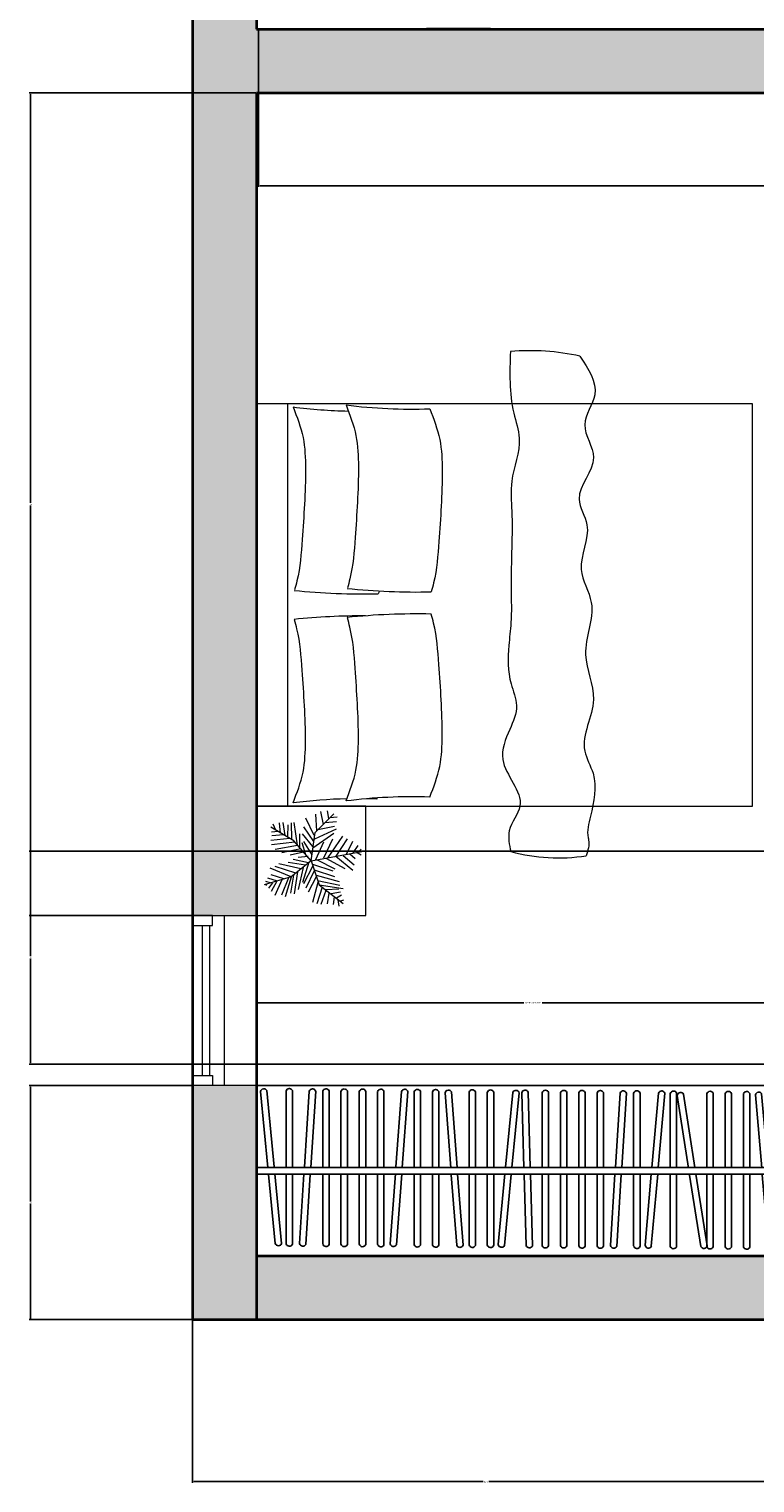
# Model space of a CAD drawing. Units: inches. Extents: x 1789 to 2841, y 3180 to 3702.
# Tile 8 of 14: x 2374 to 2477, y 3180 to 3385. Entities that reach past the tile are written whole.
import ezdxf

# ---------------------------------------------------------------- set-up
doc = ezdxf.new("R2010")
doc.units = ezdxf.units.IN
doc.header["$MEASUREMENT"] = 0
for name, color, linetype, lineweight in [('A-ANNO-DIMS', 2, 'Continuous', 18), ('A-FLOR-CASE', 34, 'Continuous', 25), ('A-WALL', 40, 'Continuous', 35), ('A-WALL-PATT', 252, 'Continuous', 13), ('FURNITURE', 34, 'Continuous', 18), ('WINDOWS', 130, 'Continuous', 18)]:
    doc.layers.add(name, color=color, linetype=linetype, lineweight=lineweight)
doc.styles.get("Standard").update_dxf_attribs({"font": 'arial.ttf'})
doc.dimstyles.get("Standard").update_dxf_attribs({"dimtxt": 0.18, "dimasz": 0.18, "dimexe": 0.18, "dimexo": 0.0625, "dimgap": 0.09, "dimtad": 0, "dimtih": 1, "dimtoh": 1, "dimdec": 0, "dimzin": 0, "dimdsep": 46, "dimlunit": 3, "dimtxsty": 'Standard', "dimcen": 0.09, "dimadec": 0, "dimazin": 0, "dimtfac": 1, "dimtdec": 0, "dimtofl": 0, "dimtmove": 0, "dimatfit": 3, "dimfxl": 1, "dimtolj": 1, "dimtzin": 0, "dimarcsym": 0})

# ---------------------------------------------------------------- blocks, each defined once
blk = doc.blocks.new('CUBOARD')
for p, q in [((2183.73, 3646.16), (2183.73, 3568.16)), ((2184.71, 3646.16), (2184.71, 3568.16))]:
    blk.add_line(p, q)
blk.add_lwpolyline([(2172.23, 3646.16), (2196.23, 3646.16), (2196.23, 3568.16), (2172.23, 3568.16)], close=True)
for points in [[(2195.39, 3645.6), (2184.67, 3644.55)], [(2183.69, 3644.46), (2173.95, 3643.51)], [(2173.97, 3642.61), (2183.78, 3643.57)], [(2184.76, 3643.66), (2195.54, 3644.71)], [(2195.78, 3645.16), (2195.78, 3645.18)], [(2183.73, 3641.98), (2173.93, 3641.98)], [(2195.47, 3641.98), (2184.71, 3641.98)], [(2195.82, 3641.5), (2195.82, 3641.53)], [(2173.86, 3641.08), (2183.73, 3641.08)], [(2183.76, 3639.46), (2173.96, 3640.08)], [(2184.71, 3641.08), (2195.53, 3641.08)], [(2195.45, 3638.71), (2184.74, 3639.4)], [(2173.84, 3639.19), (2183.7, 3638.57)], [(2184.68, 3638.5), (2195.46, 3637.81)], [(2195.77, 3638.22), (2195.78, 3638.24)], [(2173.83, 3635.92), (2183.73, 3635.92)], [(2183.73, 3636.82), (2173.9, 3636.82)], [(2195.43, 3636.82), (2184.71, 3636.82)], [(2184.71, 3635.92), (2195.5, 3635.92)], [(2195.78, 3636.35), (2195.78, 3636.37)], [(2173.81, 3633.34), (2183.73, 3633.34)], [(2183.73, 3634.24), (2173.88, 3634.24)], [(2195.42, 3634.24), (2184.71, 3634.24)], [(2184.71, 3633.34), (2195.48, 3633.34)], [(2195.77, 3633.77), (2195.77, 3633.79)], [(2183.73, 3631.66), (2173.86, 3631.66)], [(2195.4, 3631.66), (2184.71, 3631.66)], [(2195.75, 3631.19), (2195.75, 3631.21)], [(2173.8, 3630.76), (2183.73, 3630.76)], [(2184.71, 3630.76), (2195.47, 3630.76)], [(2173.78, 3628.19), (2183.73, 3628.19)], [(2183.73, 3629.08), (2173.85, 3629.08)], [(2183.8, 3626.57), (2173.93, 3627.31)], [(2195.38, 3629.08), (2184.71, 3629.08)], [(2184.71, 3628.19), (2195.45, 3628.19)], [(2195.73, 3628.61), (2195.73, 3628.63)], [(2173.79, 3626.43), (2183.74, 3625.68)], [(2184.71, 3625.61), (2195.4, 3624.81)], [(2195.4, 3625.7), (2184.78, 3626.5)], [(2195.72, 3625.21), (2195.72, 3625.23)], [(2173.75, 3623.03), (2183.73, 3623.03)], [(2183.73, 3623.92), (2173.81, 3623.92)], [(2195.35, 3623.92), (2184.71, 3623.92)], [(2184.71, 3623.03), (2195.42, 3623.03)], [(2195.7, 3623.45), (2195.7, 3623.48)], [(2183.73, 3621.34), (2173.8, 3621.34)], [(2195.33, 3621.34), (2184.71, 3621.34)], [(2173.73, 3620.45), (2183.73, 3620.45)], [(2195.22, 3619.57), (2184.65, 3618.76)], [(2184.71, 3620.45), (2195.4, 3620.45)], [(2195.6, 3619.13), (2195.6, 3619.15)], [(2195.68, 3620.87), (2195.68, 3620.9)], [(2183.67, 3618.69), (2173.75, 3617.93)], [(2173.75, 3617.03), (2183.74, 3617.8)], [(2184.71, 3617.87), (2195.35, 3618.68)], [(2173.7, 3615.29), (2183.73, 3615.29)], [(2183.73, 3616.19), (2173.77, 3616.19)], [(2195.3, 3616.19), (2184.71, 3616.19)], [(2184.71, 3615.29), (2195.37, 3615.29)], [(2195.65, 3615.71), (2195.65, 3615.74)], [(2173.68, 3612.71), (2183.73, 3612.71)], [(2183.73, 3613.61), (2173.75, 3613.61)], [(2195.28, 3613.61), (2184.71, 3613.61)], [(2184.71, 3612.71), (2195.35, 3612.71)], [(2195.63, 3613.14), (2195.63, 3613.16)], [(2173.67, 3611.18), (2183.69, 3610.23)], [(2183.78, 3611.12), (2173.82, 3612.07)], [(2195.26, 3610.03), (2184.75, 3611.03)], [(2184.67, 3610.14), (2195.24, 3609.13)], [(2195.23, 3608.76), (2184.7, 3608.45)], [(2195.56, 3609.53), (2195.57, 3609.55)], [(2173.66, 3607.23), (2183.75, 3607.53)], [(2183.72, 3608.42), (2173.71, 3608.13)], [(2184.73, 3607.55), (2195.33, 3607.87)], [(2195.6, 3608.3), (2195.6, 3608.32)], [(2173.63, 3604.98), (2183.73, 3604.98)], [(2183.73, 3605.87), (2173.7, 3605.87)], [(2195.23, 3605.87), (2184.71, 3605.87)], [(2184.71, 3604.98), (2195.3, 3604.98)], [(2195.58, 3605.4), (2195.58, 3605.42)], [(2183.73, 3603.29), (2173.68, 3603.29)], [(2195.22, 3603.29), (2184.71, 3603.29)], [(2195.57, 3602.82), (2195.57, 3602.84)], [(2173.61, 3602.4), (2183.73, 3602.4)], [(2183.73, 3600.71), (2173.67, 3600.71)], [(2184.71, 3602.4), (2195.28, 3602.4)], [(2195.2, 3600.71), (2184.71, 3600.71)], [(2173.6, 3599.82), (2183.73, 3599.82)], [(2184.71, 3599.82), (2195.27, 3599.82)], [(2195.55, 3600.24), (2195.55, 3600.27)], [(2173.58, 3597.24), (2183.73, 3597.24)], [(2183.73, 3598.13), (2173.65, 3598.13)], [(2195.18, 3598.13), (2184.71, 3598.13)], [(2184.71, 3597.24), (2195.25, 3597.24)], [(2195.53, 3597.66), (2195.53, 3597.69)], [(2173.56, 3595.36), (2183.71, 3594.72)], [(2183.77, 3595.62), (2173.68, 3596.25)], [(2184.69, 3594.66), (2195.19, 3594)], [(2195.18, 3594.9), (2184.74, 3595.55)], [(2195.5, 3594.4), (2195.5, 3594.43)], [(2183.73, 3592.98), (2173.62, 3592.98)], [(2195.15, 3592.98), (2184.71, 3592.98)], [(2195.5, 3592.5), (2195.5, 3592.53)], [(2173.55, 3592.08), (2183.73, 3592.08)], [(2173.57, 3590.49), (2183.74, 3589.59)], [(2183.73, 3590.49), (2173.72, 3591.37)], [(2184.71, 3592.08), (2195.22, 3592.08)], [(2195.17, 3589.47), (2184.71, 3590.4)], [(2184.71, 3589.5), (2195.16, 3588.58)], [(2195.48, 3588.97), (2195.48, 3589)], [(2173.51, 3586.92), (2183.73, 3586.92)], [(2183.73, 3587.82), (2173.58, 3587.82)], [(2194.84, 3586.83), (2184.58, 3585.23)], [(2195.12, 3587.82), (2184.71, 3587.82)], [(2184.71, 3586.92), (2195.19, 3586.92)], [(2195.26, 3586.41), (2195.25, 3586.44)], [(2195.47, 3587.35), (2195.47, 3587.37)], [(2183.61, 3585.08), (2173.56, 3583.51)], [(2173.63, 3582.62), (2183.75, 3584.19)], [(2184.71, 3584.34), (2195.04, 3585.95)], [(2183.73, 3582.66), (2173.55, 3582.66)], [(2195.08, 3582.66), (2184.71, 3582.66)], [(2195.43, 3582.19), (2195.43, 3582.21)], [(2173.48, 3581.77), (2183.73, 3581.77)], [(2183.73, 3580.08), (2173.53, 3580.08)], [(2184.71, 3581.77), (2195.15, 3581.77)], [(2195.07, 3580.08), (2184.71, 3580.08)], [(2173.46, 3579.19), (2183.73, 3579.19)], [(2184.71, 3579.19), (2195.14, 3579.19)], [(2195.42, 3579.61), (2195.42, 3579.63)], [(2173.45, 3576.61), (2183.73, 3576.61)], [(2183.73, 3577.5), (2173.52, 3577.5)], [(2194.92, 3575.81), (2184.64, 3574.92)], [(2195.05, 3577.5), (2184.71, 3577.5)], [(2184.71, 3576.61), (2195.12, 3576.61)], [(2195.4, 3577.03), (2195.4, 3577.05)], [(2183.66, 3574.84), (2173.46, 3573.95)], [(2173.47, 3573.05), (2183.74, 3573.94)], [(2184.71, 3574.03), (2195.06, 3574.93)], [(2195.31, 3575.37), (2195.31, 3575.4)], [(2183.65, 3572.24), (2173.45, 3571.25)], [(2194.88, 3573.34), (2184.63, 3572.34)], [(2184.71, 3571.45), (2195.04, 3572.46)], [(2195.28, 3572.91), (2195.27, 3572.93)], [(2173.47, 3570.35), (2183.74, 3571.35)], [(2183.73, 3569.77), (2173.47, 3569.77)], [(2195, 3569.77), (2184.71, 3569.77)], [(2173.4, 3568.87), (2183.73, 3568.87)], [(2184.71, 3568.87), (2195.07, 3568.87)], [(2195.35, 3569.29), (2195.35, 3569.32)]]:
    blk.add_lwpolyline(points)
for centre, start, end in [((2195.31, 3645.13), 7.0195, 80.386), ((2174.12, 3643.06), 110.7367, 251.6587), ((2195.31, 3645.13), 299.464, 4.1032), ((2174.06, 3641.52), 105.1753, 246.0974), ((2195.34, 3641.52), 1.4582, 74.8247), ((2195.34, 3641.52), 293.9026, 358.5418), ((2174.06, 3639.62), 101.5232, 242.4452), ((2195.3, 3638.26), 357.8061, 71.1726), ((2195.3, 3638.26), 290.2505, 354.8897), ((2174.02, 3636.36), 105.1753, 246.0974), ((2195.31, 3636.36), 1.4582, 74.8247), ((2195.31, 3636.36), 293.9026, 358.5418), ((2174.01, 3633.78), 105.1753, 246.0974), ((2195.29, 3633.78), 1.4582, 74.8247), ((2195.29, 3633.78), 293.9026, 358.5418), ((2173.99, 3631.2), 105.1753, 246.0974), ((2195.27, 3631.2), 1.4582, 74.8247), ((2195.27, 3631.2), 293.9026, 358.5418), ((2173.97, 3628.62), 105.1753, 246.0974), ((2174.02, 3626.85), 100.888, 241.81), ((2195.26, 3628.62), 1.4582, 74.8247), ((2195.26, 3628.62), 293.9026, 358.5418), ((2195.24, 3625.25), 357.1709, 70.5374), ((2195.24, 3625.25), 289.6153, 354.2545), ((2173.94, 3623.46), 105.1753, 246.0974), ((2195.22, 3623.46), 1.4582, 74.8247), ((2195.22, 3623.46), 293.9026, 358.5418), ((2173.92, 3620.88), 105.1753, 246.0974), ((2195.21, 3620.88), 1.4582, 74.8247), ((2195.13, 3619.1), 5.8369, 79.2034), ((2195.13, 3619.1), 298.2814, 2.9206), ((2195.21, 3620.88), 293.9026, 358.5418), ((2173.9, 3617.48), 109.5541, 250.4761), ((2173.89, 3615.73), 105.1753, 246.0974), ((2195.17, 3615.73), 1.4582, 74.8247), ((2195.17, 3615.73), 293.9026, 358.5418), ((2173.87, 3613.15), 105.1753, 246.0974), ((2195.16, 3613.15), 1.4582, 74.8247), ((2195.16, 3613.15), 293.9026, 358.5418), ((2173.9, 3611.6), 99.7479, 240.6699), ((2195.12, 3608.3), 3.1408, 76.5073), ((2195.09, 3609.58), 288.4752, 353.1144), ((2195.09, 3609.58), 356.0307, 69.3973), ((2173.84, 3607.67), 106.858, 247.78), ((2195.12, 3608.3), 295.5853, 0.2245), ((2173.82, 3605.41), 105.1753, 246.0974), ((2195.11, 3605.41), 1.4582, 74.8247), ((2195.11, 3605.41), 293.9026, 358.5418), ((2173.81, 3602.83), 105.1753, 246.0974), ((2195.09, 3602.83), 1.4582, 74.8247), ((2195.09, 3602.83), 293.9026, 358.5418), ((2173.79, 3600.25), 105.1753, 246.0974), ((2195.08, 3600.25), 1.4582, 74.8247), ((2195.08, 3600.25), 293.9026, 358.5418), ((2173.77, 3597.67), 105.1753, 246.0974), ((2195.06, 3597.67), 1.4582, 74.8247), ((2195.06, 3597.67), 293.9026, 358.5418), ((2173.78, 3595.78), 101.566, 242.4881), ((2195.02, 3594.44), 357.8489, 71.2154), ((2195.02, 3594.44), 290.2933, 354.9325), ((2173.74, 3592.52), 105.1753, 246.0974), ((2195.03, 3592.52), 1.4582, 74.8247), ((2195.03, 3592.52), 293.9026, 358.5418), ((2173.8, 3590.9), 100.1162, 241.0382), ((2195.01, 3589.03), 288.8435, 353.4827), ((2195.01, 3589.03), 356.399, 69.7655), ((2173.71, 3587.36), 105.1753, 246.0974), ((2194.79, 3586.35), 10.3063, 83.6728), ((2194.79, 3586.35), 302.7507, 7.3899), ((2194.99, 3587.36), 1.4582, 74.8247), ((2194.99, 3587.36), 293.9026, 358.5418), ((2173.67, 3582.2), 105.1753, 246.0974), ((2173.75, 3583.08), 114.0234, 254.9455), ((2194.96, 3582.2), 1.4582, 74.8247), ((2194.96, 3582.2), 293.9026, 358.5418), ((2173.66, 3579.62), 105.1753, 246.0974), ((2194.94, 3579.62), 1.4582, 74.8247), ((2194.94, 3579.62), 293.9026, 358.5418), ((2173.64, 3577.04), 105.1753, 246.0974), ((2194.83, 3575.34), 6.4142, 79.7807), ((2194.93, 3577.04), 1.4582, 74.8247), ((2194.93, 3577.04), 293.9026, 358.5418), ((2173.63, 3573.5), 110.1314, 251.0534), ((2194.83, 3575.34), 298.8587, 3.4979), ((2194.8, 3572.87), 7.0476, 80.4142), ((2194.8, 3572.87), 299.4921, 4.1313), ((2173.59, 3569.31), 105.1753, 246.0974), ((2173.62, 3570.8), 110.7648, 251.6868), ((2194.88, 3569.31), 1.4582, 74.8247), ((2194.88, 3569.31), 293.9026, 358.5418)]:
    blk.add_arc(centre, 0.476, start, end)
blk = doc.blocks.new('HY')
for p, q in [((2053.67, 3653.75), (2074.8, 3653.75)), ((2053.67, 3652.75), (2074.8, 3652.75)), ((2052.23, 3650.66), (2076.23, 3650.66))]:
    blk.add_line(p, q)
for points in [[(2076.23, 3646.16), (2052.23, 3646.16), (2052.23, 3655.16), (2076.23, 3655.16)], [(2052.23, 3655.16), (2053.67, 3655.16), (2053.67, 3652.35), (2052.23, 3652.35)], [(2076.23, 3655.16), (2074.8, 3655.16), (2074.8, 3652.35), (2076.23, 3652.35)]]:
    blk.add_lwpolyline(points, close=True)
blk = doc.blocks.new('*U22')
for p, q in [((-8.737, 47.138), (-17.069, 52.711)), ((-10.186, 53.64), (-13.084, 55.962)), ((0, 0), (-10.5, 57)), ((-9.099, 51.782), (-6.563, 55.962)), ((-7.65, 43.423), (-2.578, 49.46)), ((-3.665, 19.273), (-27.574, 35.527)), ((-5.114, 28.097), (-24.676, 40.636)), ((-7.288, 39.707), (-21.778, 46.673)), ((-5.839, 35.992), (4.667, 48.067)), ((-5.114, 27.632), (10.463, 46.673)), ((-2.941, 16.486), (8.652, 37.85)), ((27, 9), (48, 36)), ((27.127, 9.056), (31.112, 35.992)), ((35.096, 32.741), (37.27, 22.524)), ((38.719, 34.134), (41.979, 28.561)), ((44.153, 36.456), (45.239, 32.741)), ((-47.498, 19.737), (-55.83, 18.344)), ((-31.5, 4.5), (-52.5, 25.5)), ((-48.585, 21.131), (-49.309, 29.026)), ((-43.513, 28.561), (-42.427, 15.558)), ((-38.442, 26.239), (-34.819, 7.663)), ((-35.544, 28.097), (-24.314, 3.947)), ((-14.533, 2.09), (-30.834, 25.31)), ((-24.314, 23.917), (-2.941, 13.7)), ((-1.129, 6.734), (9.014, 26.704)), ((3.942, 1.625), (11.187, 24.381)), ((10.101, 3.483), (17.708, 26.239)), ((16.259, 5.805), (23.142, 31.348)), ((22.055, 7.198), (27.489, 32.277)), ((31.836, 30.883), (32.561, 16.486)), ((33.285, 16.486), (48.862, 10.913)), ((36.183, 19.737), (48.137, 17.88)), ((40.53, 25.775), (48.862, 24.846)), ((43.791, 29.954), (51.036, 30.883)), ((-40.615, 13.7), (-55.105, 10.913)), ((-33.37, 6.269), (-52.207, 5.34)), ((-28.299, 3.483), (-47.86, -5.805)), ((-21.416, 3.018), (-38.079, -8.128)), ((0, 0), (-31.5, 4.5)), ((-15.982, 2.09), (-30.11, -9.521)), ((0, 0), (-22.5, -19.5)), ((-6.563, 1.161), (-21.416, -8.128)), ((-20.691, 13.7), (-1.129, 4.876)), ((0, 0), (27, 9)), ((0, 0), (18, -22.5)), ((6.478, 1.625), (26.04, -8.592)), ((11.187, 3.483), (30.749, -5.805)), ((18.07, 5.805), (35.096, -3.483)), ((24.229, 7.663), (46.688, 1.625)), ((29.662, 12.307), (48.137, 6.269)), ((-17.431, -15.094), (-42.789, -18.809)), ((-15.257, -12.772), (-30.11, -12.772)), ((-6.563, -5.805), (-19.967, -9.985)), ((-17.069, -15.094), (-12.721, -40.172)), ((-13.446, -11.378), (-8.737, -32.741)), ((-9.461, -8.592), (-6.201, -23.453)), ((-4.752, -3.483), (-3.665, -14.629)), ((2.493, -3.019), (-1.491, -20.202)), ((1.769, -2.555), (24.229, -9.521)), ((5.029, -6.27), (2.131, -25.775)), ((9.014, -11.378), (3.58, -35.992)), ((7.565, -9.056), (32.198, -14.629)), ((12.274, -15.094), (36.907, -18.809)), ((-28.299, -29.026), (-42.789, -31.348)), ((-24.314, -21.596), (-42.427, -22.06)), ((-26.849, -26.24), (-40.253, -25.775)), ((-22.5, -19.5), (-37.5, -45)), ((-29.023, -30.884), (-27.936, -43.887)), ((-25.038, -23.918), (-22.865, -45.281)), ((-20.691, -18.345), (-17.793, -44.352)), ((14.085, -16.951), (6.478, -40.172)), ((18.07, -22.524), (8.289, -45.745)), ((20.244, -30.419), (15.897, -44.816)), ((16.259, -19.738), (36.183, -22.989)), ((18, -22.5), (27, -52.5)), ((18.433, -22.524), (40.53, -29.026)), ((19.157, -25.311), (38.719, -33.206)), ((-30.834, -34.135), (-42.427, -35.528)), ((-34.457, -39.708), (-40.978, -42.494)), ((-32.646, -36.921), (-31.921, -44.352)), ((22.78, -37.85), (19.519, -48.532)), ((21.331, -32.741), (39.081, -40.636)), ((22.78, -38.314), (34.372, -44.816)), ((24.591, -45.745), (23.142, -50.854)), ((24.591, -43.423), (30.749, -47.603)), ((26.764, -49.925), (28.213, -50.854))]:
    blk.add_line(p, q)
blk = doc.blocks.new('BEDD')
for points in [[(2235.4, 3526.16), (2292.14, 3526.16), (2292.14, 3596.12), (2235.4, 3596.12)], [(2292.14, 3526.16), (2307.57, 3526.16), (2307.57, 3541.59), (2292.14, 3541.59)], [(2235.4, 3526.16), (2292.14, 3526.16), (2292.14, 3530.61), (2235.4, 3530.61)]]:
    blk.add_lwpolyline(points, close=True)
for centre, radius, start, end in [((2259.99, 3564.78), 32.07, 167.4063, 185.0216), ((2273.81, 3568.71), 25.64, 344.9042, 8.8372), ((2163.47, 3548.06), 72.69, 352.674, 2.0029), ((2165.57, 3548.81), 96.38, 354.1175, 1.1854), ((2361.42, 3548.81), 96.38, 178.8146, 185.8825), ((2363.52, 3548.06), 72.69, 177.9971, 187.326), ((2165.85, 3541.35), 96.38, 354.1175, 1.1854), ((2363.79, 3540.6), 72.69, 177.9971, 179.1531), ((2361.69, 3541.35), 96.38, 179.877, 185.8825), ((2163.75, 3540.6), 72.69, 352.674, 358.8312), ((2363.79, 3540.6), 72.69, 181.3344, 187.326)]:
    blk.add_arc(centre, radius, start, end)
for points, knots in [([(2228.7, 3571.77), (2230.5, 3572.97), (2233.69, 3575.11), (2238.44, 3571.24), (2243.48, 3575.3), (2248.08, 3570.3), (2253.24, 3573.93), (2258.37, 3570.76), (2264.15, 3574.63), (2270.52, 3571.37), (2277.36, 3575.01), (2283.2, 3571.25), (2288.29, 3574.45), (2292.59, 3573.51), (2295.73, 3572.7), (2297.56, 3573.17), (2298.4, 3572.89), (2299.15, 3572.65)], [0, 0, 0, 0, 5.813057, 10.291797, 15.071674, 21.264477, 25.062958, 31.395117, 36.284741, 43.6566, 50.0956, 57.47363, 60.824937, 66.871309, 69.965772, 70.260383, 72.512122, 72.512122, 72.512122, 72.512122]), ([(2228.05, 3561.97), (2230.96, 3561.87), (2235.09, 3561.73), (2241.08, 3563.86), (2245.67, 3561.8), (2250.85, 3562.25), (2255.91, 3562.17), (2261.15, 3562), (2265.78, 3562.19), (2270.21, 3561.59), (2274.18, 3561.57), (2278.08, 3563.31), (2281.58, 3561.74), (2286.46, 3559.73), (2291.21, 3564.99), (2295.28, 3561.31), (2297.57, 3561.81), (2298.57, 3562.03)], [0, 0, 0, 0, 8.669632, 12.310458, 18.461416, 22.693385, 27.790985, 33.658819, 38.43562, 41.630677, 47.052462, 50.224855, 53.725722, 58.058029, 65.069701, 68.862462, 71.815525, 71.815525, 71.815525, 71.815525]), ([(2236.12, 3550.6), (2237.54, 3551.15), (2240.34, 3552.23), (2246.72, 3552.46), (2253.43, 3551.99), (2259.2, 3551.57), (2261.51, 3550.92), (2261.93, 3550.8)], [0, 0, 0, 0, 4.544245, 8.926813, 18.957656, 24.819591, 26.148375, 26.148375, 26.148375, 26.148375]), ([(2290.87, 3550.6), (2289.45, 3551.15), (2286.65, 3552.23), (2280.27, 3552.46), (2273.56, 3551.99), (2267.8, 3551.57), (2265.49, 3550.92), (2265.06, 3550.8)], [0, 0, 0, 0, 4.544245, 8.926813, 18.957656, 24.819591, 26.148375, 26.148375, 26.148375, 26.148375]), ([(2235.57, 3538.79), (2236.99, 3539.34), (2239.79, 3540.42), (2246.18, 3540.65), (2252.88, 3540.18), (2258.65, 3539.76), (2260.96, 3539.11), (2261.38, 3538.99)], [0, 0, 0, 0, 4.544245, 8.926813, 18.957656, 24.819591, 26.148375, 26.148375, 26.148375, 26.148375]), ([(2291.42, 3538.79), (2290, 3539.34), (2287.2, 3540.42), (2280.82, 3540.65), (2274.11, 3540.18), (2268.34, 3539.76), (2266.03, 3539.11), (2265.61, 3538.99)], [0, 0, 0, 0, 4.544245, 8.926813, 18.957656, 24.819591, 26.148375, 26.148375, 26.148375, 26.148375]), ([(2235.84, 3531.33), (2237.27, 3531.88), (2240.06, 3532.96), (2246.45, 3533.19), (2253.15, 3532.71), (2258.92, 3532.3), (2261.23, 3531.65), (2261.66, 3531.53)], [0, 0, 0, 0, 4.544245, 8.926813, 18.957656, 24.819591, 26.148375, 26.148375, 26.148375, 26.148375]), ([(2291.69, 3531.33), (2290.27, 3531.88), (2287.47, 3532.96), (2281.09, 3533.19), (2274.39, 3532.71), (2268.62, 3532.3), (2266.31, 3531.65), (2265.88, 3531.53)], [0, 0, 0, 0, 4.544245, 8.926813, 18.957656, 24.819591, 26.148375, 26.148375, 26.148375, 26.148375])]:
    blk.add_open_spline(points, degree=3, knots=knots)
for points in [[(2261.81, 3543.46), (2261.94, 3543.42), (2262.07, 3543.38), (2262.21, 3543.34)], [(2291.15, 3543.14), (2291.09, 3543.16), (2291.04, 3543.18), (2290.99, 3543.2)]]:
    blk.add_open_spline(points, degree=3)
at = {"xscale": 0.1258179792922857, "yscale": 0.1258179792922857, "zscale": 0.1258179792922857}
blk.add_blockref('*U22', (2299.85, 3533.87), dxfattribs=at)
blk = doc.blocks.new('*D37')
at = {"layer": 'A-ANNO-DIMS', "color": 0, "lineweight": -2, "transparency": 16777216}
for p, q in [((2406.23, 3236.22), (2406.23, 3248.04)), ((2406.41, 3247.86), (2443.93, 3247.86)), ((2484.05, 3247.86), (2446.54, 3247.86)), ((2484.23, 3236.22), (2484.23, 3248.04))]:
    blk.add_line(p, q, dxfattribs=at)
at = {"layer": 'A-ANNO-DIMS', "color": 0, "transparency": 16777216}
for points in [[(2406.41, 3247.89), (2406.41, 3247.83), (2406.23, 3247.86)], [(2484.05, 3247.89), (2484.05, 3247.83), (2484.23, 3247.86)]]:
    blk.add_solid(points, dxfattribs=at)
at = {"layer": 'Defpoints', "color": 0, "transparency": 16777216}
for p in [(2406.23, 3247.86), (2406.23, 3236.16), (2484.23, 3236.16)]:
    blk.add_point(p, dxfattribs=at)
at = {"layer": 'A-ANNO-DIMS', "color": 0, "transparency": 16777216, "insert": (2445.23, 3247.86), "char_height": 0.18, "attachment_point": 5}
blk.add_mtext('\\A1;WARDROBE 78 TYP.', dxfattribs=at)
blk = doc.blocks.new('*D69')
at = {"layer": 'A-ANNO-DIMS', "color": 0, "lineweight": -2, "transparency": 16777216}
for p, q in [((2406.54, 3385.11), (2406.54, 3362.9)), ((2553.79, 3385.11), (2553.79, 3362.9)), ((2406.72, 3363.08), (2478.8, 3363.08)), ((2553.61, 3363.08), (2481.54, 3363.08))]:
    blk.add_line(p, q, dxfattribs=at)
at = {"layer": 'A-ANNO-DIMS', "color": 0, "transparency": 16777216}
for points in [[(2406.72, 3363.11), (2406.72, 3363.05), (2406.54, 3363.08)], [(2553.61, 3363.11), (2553.61, 3363.05), (2553.79, 3363.08)]]:
    blk.add_solid(points, dxfattribs=at)
at = {"layer": 'Defpoints', "color": 0, "transparency": 16777216}
for p in [(2406.54, 3385.17), (2553.79, 3385.17), (2553.79, 3363.08)]:
    blk.add_point(p, dxfattribs=at)
at = {"layer": 'A-ANNO-DIMS', "color": 0, "transparency": 16777216, "insert": (2480.17, 3363.08), "char_height": 0.18, "attachment_point": 5}
blk.add_mtext('\\A1;SEATING GROUP 147', dxfattribs=at)
blk = doc.blocks.new('*D97')
at = {"layer": 'A-ANNO-DIMS', "color": 0, "lineweight": -2, "transparency": 16777216}
for p, q in [((2397.23, 3203.1), (2397.23, 3180.13)), ((2479.95, 3203.1), (2479.95, 3180.13)), ((2397.41, 3180.31), (2438.2, 3180.31)), ((2479.77, 3180.31), (2438.98, 3180.31))]:
    blk.add_line(p, q, dxfattribs=at)
at = {"layer": 'A-ANNO-DIMS', "color": 0, "transparency": 16777216}
for points in [[(2397.41, 3180.34), (2397.41, 3180.28), (2397.23, 3180.31)], [(2479.77, 3180.34), (2479.77, 3180.28), (2479.95, 3180.31)]]:
    blk.add_solid(points, dxfattribs=at)
at = {"layer": 'Defpoints', "color": 0, "transparency": 16777216}
for p in [(2397.23, 3203.16), (2479.95, 3203.16), (2479.95, 3180.31)]:
    blk.add_point(p, dxfattribs=at)
at = {"layer": 'A-ANNO-DIMS', "color": 0, "transparency": 16777216, "insert": (2438.59, 3180.31), "char_height": 0.18, "attachment_point": 5}
blk.add_mtext('\\A1;82.72', dxfattribs=at)
blk = doc.blocks.new('*D105')
at = {"layer": 'A-ANNO-DIMS', "color": 0, "lineweight": -2, "transparency": 16777216}
for p, q in [((2406.17, 3376.16), (2374.2, 3376.16)), ((2374.38, 3375.98), (2374.38, 3318.34)), ((2374.38, 3260.34), (2374.38, 3317.98)), ((2397.17, 3260.16), (2374.2, 3260.16))]:
    blk.add_line(p, q, dxfattribs=at)
at = {"layer": 'A-ANNO-DIMS', "color": 0, "transparency": 16777216}
for points in [[(2374.35, 3375.98), (2374.41, 3375.98), (2374.38, 3376.16)], [(2374.35, 3260.34), (2374.41, 3260.34), (2374.38, 3260.16)]]:
    blk.add_solid(points, dxfattribs=at)
at = {"layer": 'Defpoints', "color": 0, "transparency": 16777216}
for p in [(2406.23, 3376.16), (2374.38, 3260.16), (2397.23, 3260.16)]:
    blk.add_point(p, dxfattribs=at)
at = {"layer": 'A-ANNO-DIMS', "color": 0, "transparency": 16777216, "insert": (2374.38, 3318.16), "char_height": 0.18, "attachment_point": 5}
blk.add_mtext('\\A1;116', dxfattribs=at)
blk = doc.blocks.new('*D106')
at = {"layer": 'A-ANNO-DIMS', "color": 0, "lineweight": -2, "transparency": 16777216}
for p, q in [((2397.17, 3236.16), (2374.2, 3236.16)), ((2374.38, 3235.98), (2374.38, 3219.84)), ((2374.38, 3203.34), (2374.38, 3219.48)), ((2397.17, 3203.16), (2374.2, 3203.16))]:
    blk.add_line(p, q, dxfattribs=at)
at = {"layer": 'A-ANNO-DIMS', "color": 0, "transparency": 16777216}
for points in [[(2374.35, 3235.98), (2374.41, 3235.98), (2374.38, 3236.16)], [(2374.35, 3203.34), (2374.41, 3203.34), (2374.38, 3203.16)]]:
    blk.add_solid(points, dxfattribs=at)
at = {"layer": 'Defpoints', "color": 0, "transparency": 16777216}
for p in [(2397.23, 3236.16), (2374.38, 3203.16), (2397.23, 3203.16)]:
    blk.add_point(p, dxfattribs=at)
at = {"layer": 'A-ANNO-DIMS', "color": 0, "transparency": 16777216, "insert": (2374.38, 3219.66), "char_height": 0.18, "attachment_point": 5}
blk.add_mtext('\\A1;33', dxfattribs=at)
blk = doc.blocks.new('*D110')
at = {"layer": 'A-ANNO-DIMS', "color": 0, "lineweight": -2, "transparency": 16777216}
for p, q in [((2550.17, 3269.21), (2374.2, 3269.21)), ((2374.38, 3269.03), (2374.38, 3254.4)), ((2374.38, 3239.39), (2374.38, 3254.03)), ((2550.17, 3239.21), (2374.2, 3239.21))]:
    blk.add_line(p, q, dxfattribs=at)
at = {"layer": 'A-ANNO-DIMS', "color": 0, "transparency": 16777216}
for points in [[(2374.35, 3269.03), (2374.41, 3269.03), (2374.38, 3269.21)], [(2374.35, 3239.39), (2374.41, 3239.39), (2374.38, 3239.21)]]:
    blk.add_solid(points, dxfattribs=at)
at = {"layer": 'Defpoints', "color": 0, "transparency": 16777216}
for p in [(2374.38, 3269.21), (2550.23, 3269.21), (2550.23, 3239.21)]:
    blk.add_point(p, dxfattribs=at)
at = {"layer": 'A-ANNO-DIMS', "color": 0, "transparency": 16777216, "insert": (2374.38, 3254.21), "char_height": 0.18, "attachment_point": 5}
blk.add_mtext('\\A1;30', dxfattribs=at)

msp = doc.modelspace()

# ---------------------------------------------------------------- hatches: boundary and pattern name
at = {"layer": 'A-WALL-PATT'}
h = msp.add_hatch(color=256, dxfattribs=at)
h.dxf.hatch_style = 1
edge = h.paths.add_edge_path()
edge.add_line((2559.2333, 3385.1608), (2442.3717, 3385.1608))
edge.add_line((2442.3717, 3385.1608), (2442.3717, 3385.1524))
edge.add_line((2442.3717, 3385.1524), (2418.8108, 3385.1608))
edge.add_line((2418.8108, 3385.1608), (2406.2333, 3385.1608))
edge.add_line((2406.2333, 3385.1608), (2406.5667, 3473.2999))
edge.add_arc((2403.2333, 3513.1608), 40, 270, 274.780192, ccw=False)
edge.add_line((2403.2333, 3473.1608), (2397.2333, 3473.1608))
edge.add_line((2397.2333, 3473.1608), (2397.2333, 3376.1608))
edge.add_line((2397.2333, 3376.1608), (2550.2333, 3376.1608))
edge.add_line((2550.2333, 3376.1608), (2550.2333, 3372.6905))
edge.add_arc((2551.7333, 3408.5966), 35.9374, 267.607822, 272.392178)
edge.add_line((2553.2333, 3372.6905), (2559.2333, 3372.6905))
edge.add_line((2559.2333, 3372.6905), (2559.2333, 3385.1608))
h = msp.add_hatch(color=256, dxfattribs=at)
h.dxf.hatch_style = 1
h.paths.add_polyline_path([(2406.2333, 3376.1608), (2397.2333, 3376.1608), (2397.2333, 3260.1608), (2406.2333, 3260.1608), (2406.2333, 3275.5886), (2406.2333, 3332.3251)])
h = msp.add_hatch(color=256, dxfattribs=at)
h.dxf.hatch_style = 1
h.paths.add_polyline_path([(2592.3707, 3212.1608), (2559.2333, 3212.1608), (2559.2333, 3216.7108), (2559.2333, 3239.3636, -0.02504709), (2556.2333, 3239.2132), (2550.2333, 3239.2132), (2550.2333, 3212.1608), (2539.9504, 3212.1608), (2539.9504, 3203.1608), (2592.3707, 3203.1608)])
h.paths.add_polyline_path([(2479.9504, 3212.1608), (2406.2333, 3212.1608), (2406.2333, 3236.1608), (2397.2333, 3236.1608), (2397.2333, 3203.1608), (2479.9504, 3203.1608)])

# ---------------------------------------------------------------- linework, layer by layer
at = {"layer": 'A-WALL'}
for p, q in [((2406.5667, 3473.2999), (2406.2333, 3385.1608)), ((2397.2333, 3473.1608), (2397.2333, 3203.1608)), ((2406.2333, 3385.1608), (2559.2333, 3385.1608)), ((2439.2333, 3385.1608), (2430.2333, 3385.1608)), ((2406.2333, 3376.1608), (2406.2333, 3212.1608)), ((2406.2333, 3376.1608), (2550.2333, 3376.1608)), ((2406.2333, 3376.1608), (2406.2333, 3203.1608)), ((2406.2333, 3212.1608), (2550.2333, 3212.1608)), ((2397.2333, 3203.1608), (2763.2333, 3203.1608))]:
    msp.add_line(p, q, dxfattribs=at)

# ---------------------------------------------------------------- block references
at = {"layer": 'A-FLOR-CASE', "rotation": 90}
msp.add_blockref('CUBOARD', (6052.3941, 1039.9274), dxfattribs=at)
at = {"layer": 'FURNITURE', "rotation": 270}
msp.add_blockref('BEDD', (-1119.9274, 5567.7261), dxfattribs=at)
at = {"layer": 'WINDOWS', "rotation": 89.99999999999999}
msp.add_blockref('HY', (6052.3941, 1183.9274), dxfattribs=at)

# ---------------------------------------------------------------- dimensions: what is measured, and where the dimension line sits
at = {"layer": 'A-ANNO-DIMS'}
dim = msp.add_linear_dim(base=(2553.7897, 3363.0817), p1=(2406.5443, 3385.1685), p2=(2553.7897, 3385.1685), text='SEATING GROUP <>', dimstyle='Standard', override={"dimdec": 0, "dimlfac": 1, "dimrnd": 0, "dimzin": 0, "dimdsep": 46, "dimlunit": 2}, dxfattribs=at)
dim.commit()
dim.dimension.update_dxf_attribs({"geometry": '*D69', "text_midpoint": (2480.167, 3363.0817)})
for base, p1, p2, picture, middle in [((2374.3833, 3260.1608), (2406.2333, 3376.1608), (2397.2333, 3260.1608), '*D105', (2374.3833, 3318.1608)), ((2374.3833, 3269.2132), (2550.2333, 3239.2132), (2550.2333, 3269.2132), '*D110', (2374.3833, 3254.2132)), ((2374.3833, 3203.1608), (2397.2333, 3236.1608), (2397.2333, 3203.1608), '*D106', (2374.3833, 3219.6608))]:
    dim = msp.add_linear_dim(base=base, p1=p1, p2=p2, angle=90, dimstyle='Standard', override={"dimdec": 0, "dimlfac": 1, "dimrnd": 0, "dimzin": 0, "dimdsep": 46, "dimlunit": 2}, dxfattribs=at)
    dim.commit()
    dim.dimension.update_dxf_attribs({"geometry": picture, "text_midpoint": middle})
dim = msp.add_linear_dim(base=(2406.2333, 3247.8608), p1=(2484.2333, 3236.1608), p2=(2406.2333, 3236.1608), angle=180, text='WARDROBE <> TYP.', dimstyle='Standard', override={"dimdec": 0, "dimlfac": 1, "dimrnd": 0, "dimzin": 0, "dimdsep": 46, "dimlunit": 2}, dxfattribs=at)
dim.commit()
dim.dimension.update_dxf_attribs({"geometry": '*D37', "text_midpoint": (2445.2333, 3247.8608)})
dim = msp.add_linear_dim(base=(2479.9504, 3180.3108), p1=(2397.2333, 3203.1608), p2=(2479.9504, 3203.1608), dimstyle='Standard', override={"dimdec": 2, "dimlfac": 1, "dimrnd": 0, "dimzin": 0, "dimdsep": 46, "dimlunit": 2}, dxfattribs=at)
dim.commit()
dim.dimension.update_dxf_attribs({"geometry": '*D97', "text_midpoint": (2438.5919, 3180.3108)})

doc.saveas('drawing.dxf')
